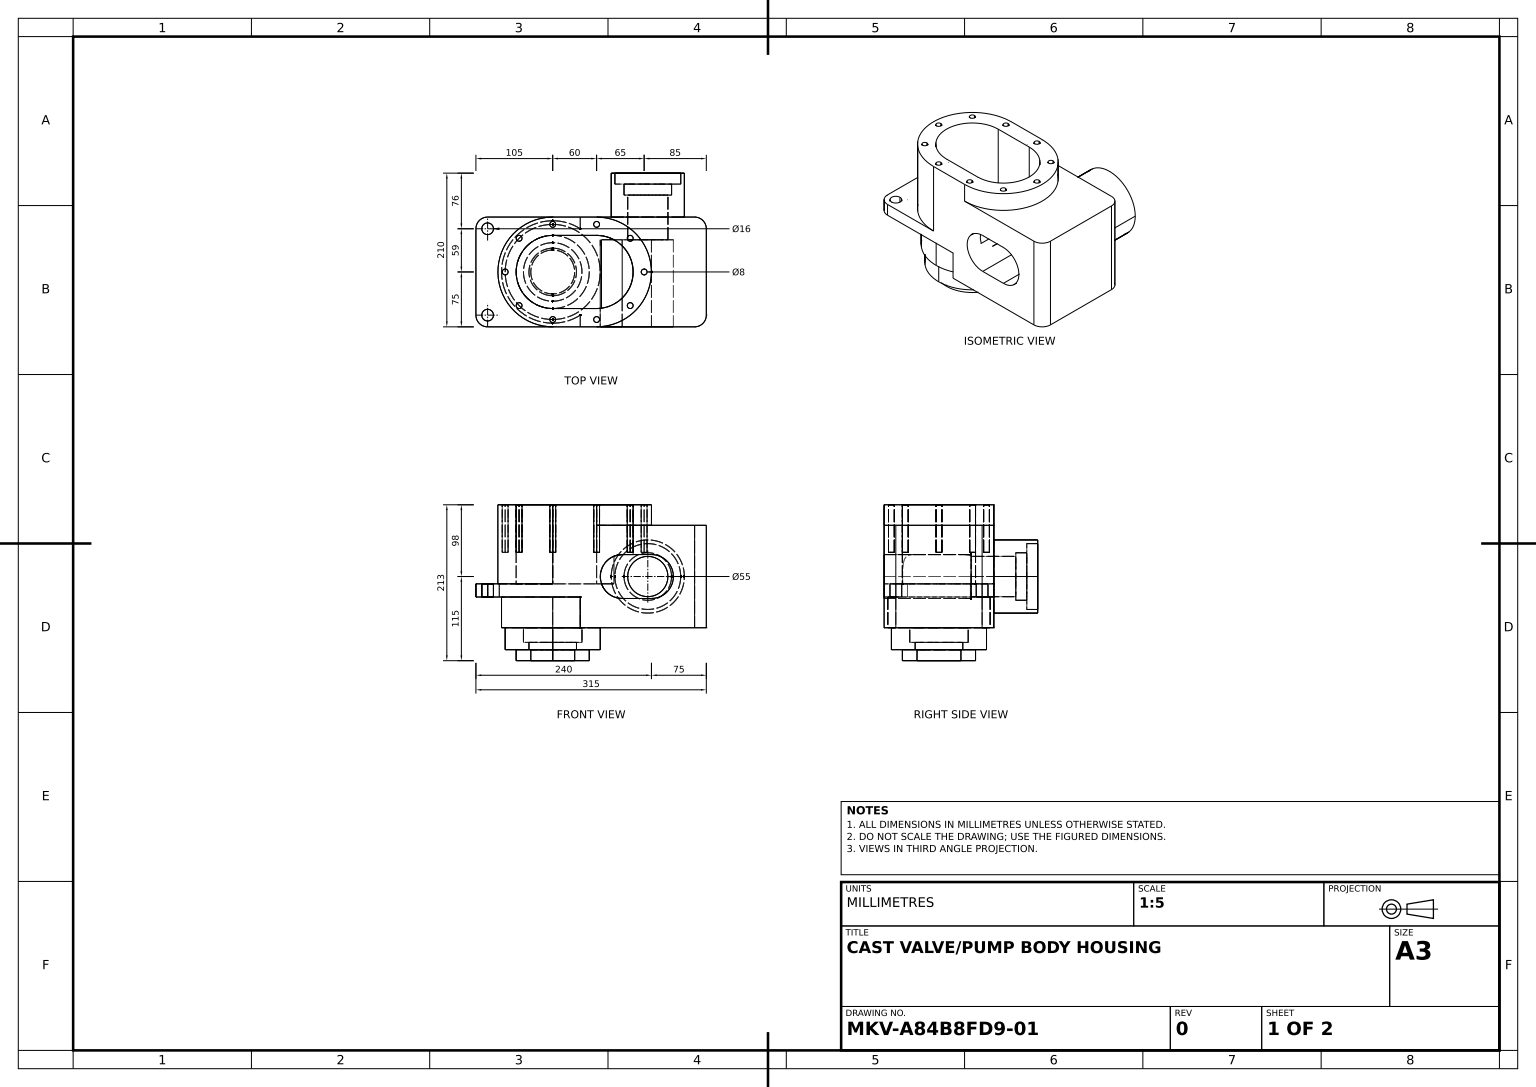
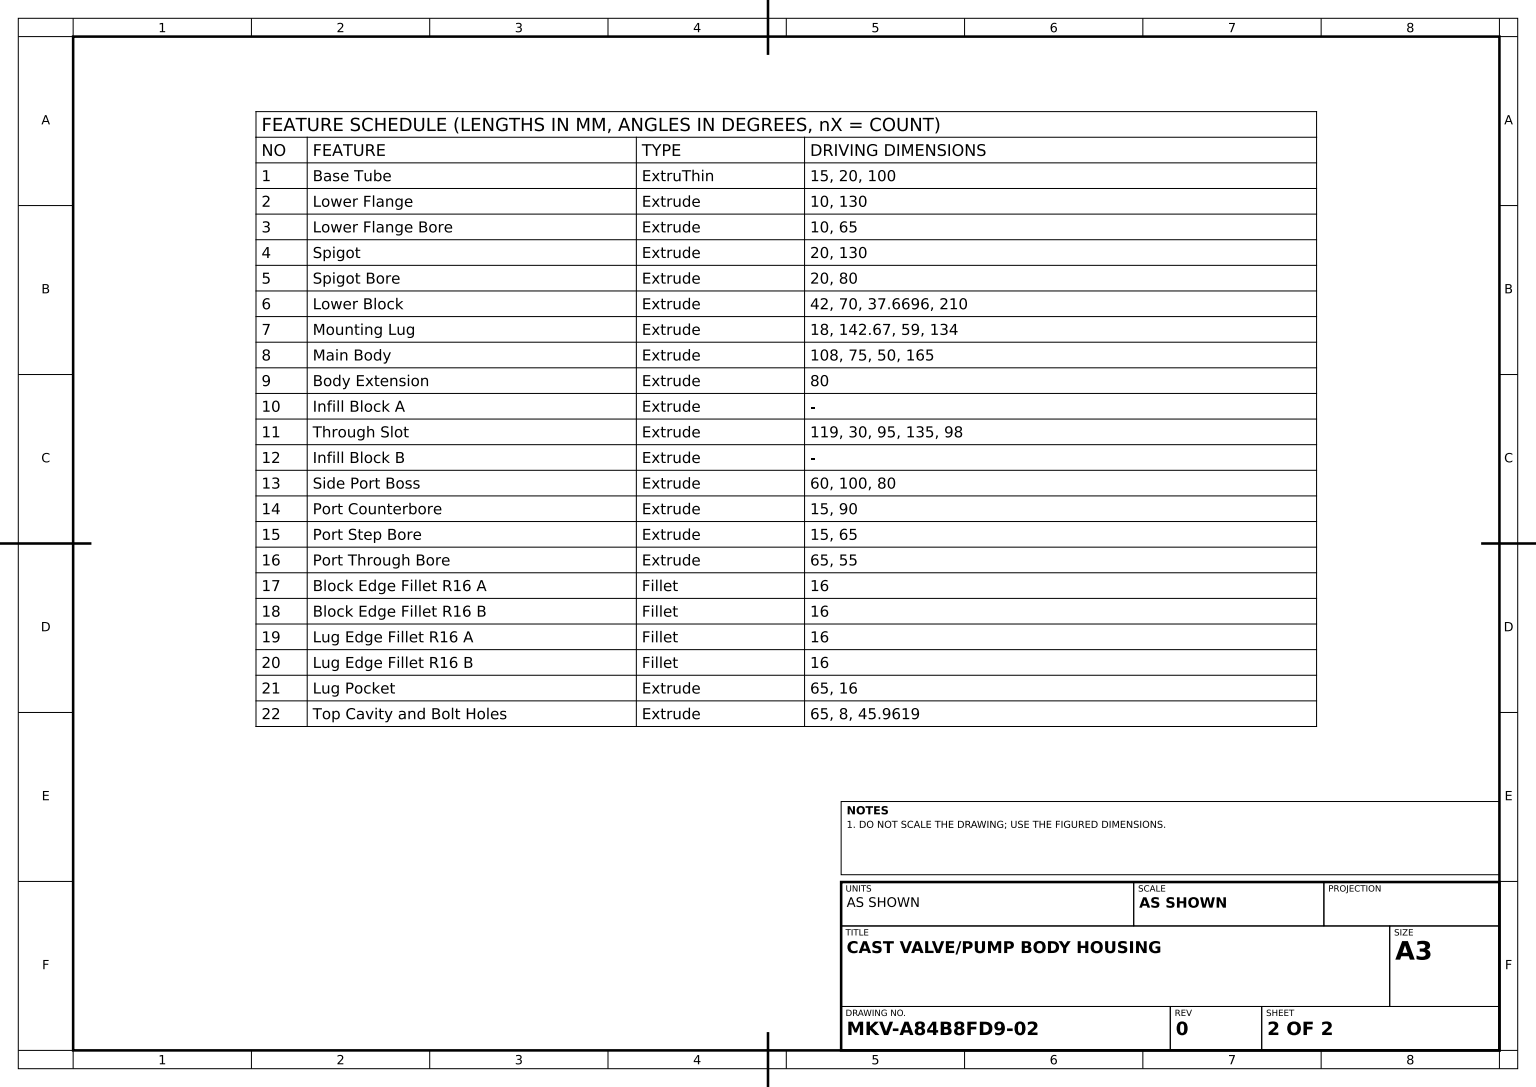
from build123d import *

# Parameters (mm, degrees)
BASE_TUBE_SKETCH_R                 = 50
BASE_TUBE_SKETCH_R_2               = 30
BASE_TUBE_DEPTH                    = 15
LOWER_FLANGE_SKETCH_R              = 65
LOWER_FLANGE_DEPTH                 = 10
LOWER_FLANGE_BORE_SKETCH_R         = 32.5
LOWER_FLANGE_BORE_DEPTH            = 10
SPIGOT_SKETCH_R                    = 65
SPIGOT_DEPTH                       = 20
SPIGOT_BORE_SKETCH_R               = 40
SPIGOT_BORE_DEPTH                  = 20
LOWER_BLOCK_DEPTH                  = 42
MOUNTING_LUG_DEPTH                 = 18
MAIN_BODY_DEPTH                    = 108
BODY_EXTENSION_DEPTH               = 80
INFILL_BLOCK_A_SKETCH_W            = 172.330383596
INFILL_BLOCK_A_SKETCH_H            = 42
INFILL_BLOCK_A_DEPTH               = 16
THROUGH_SLOT_DEPTH                 = 119
INFILL_BLOCK_B_SKETCH_W            = 172.330383596
INFILL_BLOCK_B_SKETCH_H            = 42
INFILL_BLOCK_B_DEPTH               = 16
SIDE_PORT_BOSS_SKETCH_R            = 50
SIDE_PORT_BOSS_DEPTH               = 60
PORT_COUNTERBORE_SKETCH_R          = 45
PORT_COUNTERBORE_DEPTH             = 15
PORT_STEP_BORE_SKETCH_R            = 32.5
PORT_STEP_BORE_DEPTH               = 15
PORT_THROUGH_BORE_SKETCH_R         = 27.5
PORT_THROUGH_BORE_DEPTH            = 65
BLOCK_EDGE_FILLET_R16_A_R          = 16
BLOCK_EDGE_FILLET_R16_B_R          = 16
LUG_EDGE_FILLET_R16_A_R            = 16
LUG_EDGE_FILLET_R16_B_R            = 16
LUG_POCKET_SKETCH_R                = 8
LUG_POCKET_DEPTH                   = 65
TOP_CAVITY_AND_BOLT_HOLES_SKETCH_R = 4
TOP_CAVITY_AND_BOLT_HOLES_DEPTH    = 65


with BuildPart() as part:
    # Base Tube Sketch → Base Tube (new body)
    with BuildSketch(Plane(origin=(0, 0, 0), x_dir=(1, 0, 0), z_dir=(0, 1, 0))):
        Circle(BASE_TUBE_SKETCH_R)
        Circle(BASE_TUBE_SKETCH_R_2, mode=Mode.SUBTRACT)
    extrude(amount=BASE_TUBE_DEPTH)

    # Lower Flange Sketch → Lower Flange (add)
    with BuildSketch(Plane(origin=(0, 15, 0), x_dir=(1, 0, 0), z_dir=(0, 1, 0))):
        with Locations(Location((0, 0, 0), (0, 0, 270))):
            Circle(LOWER_FLANGE_SKETCH_R)
    extrude(amount=LOWER_FLANGE_DEPTH)

    # Lower Flange Bore Sketch → Lower Flange Bore (cut)
    with BuildSketch(Plane(origin=(0, 25, 0), x_dir=(1, 0, 0), z_dir=(0, 1, 0))):
        with Locations(Location((0, 0, 0), (0, 0, 270))):
            Circle(LOWER_FLANGE_BORE_SKETCH_R)
    extrude(amount=-LOWER_FLANGE_BORE_DEPTH, mode=Mode.SUBTRACT)

    # Spigot Sketch → Spigot (add)
    with BuildSketch(Plane(origin=(0, 25, 0), x_dir=(1, 0, 0), z_dir=(0, 1, 0))):
        with Locations(Location((0, 0, 0), (0, 0, 270))):
            Circle(SPIGOT_SKETCH_R)
    extrude(amount=SPIGOT_DEPTH)

    # Spigot Bore Sketch → Spigot Bore (cut)
    with BuildSketch(Plane(origin=(0, 45, 0), x_dir=(1, 0, 0), z_dir=(0, 1, 0))):
        with Locations(Location((0, 0, 0), (0, 0, 270))):
            Circle(SPIGOT_BORE_SKETCH_R)
    extrude(amount=-SPIGOT_BORE_DEPTH, mode=Mode.SUBTRACT)

    # Lower Block Sketch → Lower Block (add)
    with BuildSketch(Plane(origin=(0, 45, 0), x_dir=(1, 0, 0), z_dir=(0, 1, 0))):
        with BuildLine():
            Line((37.669616404, 59), (210, 59))
            Line((210, 59), (210, -59))
            Line((210, -59), (37.669616404, -59))
            ThreePointArc((37.669616404, -59), (-70, 0), (37.669616404, 59))
        make_face()
    extrude(amount=LOWER_BLOCK_DEPTH)

    # Mounting Lug Sketch → Mounting Lug (add)
    with BuildSketch(Plane(origin=(0, 87, 0), x_dir=(1, 0, 0), z_dir=(0, 1, 0))):
        Polygon((-105, 0), (-105, 75), (210, 75), (210, -75), (-105, -75), align=None)
    extrude(amount=MOUNTING_LUG_DEPTH)

    # Main Body Sketch → Main Body (add)
    with BuildSketch(Plane(origin=(0, 105, 0), x_dir=(1, 0, 0), z_dir=(0, 1, 0))):
        with BuildLine():
            Line((0, 75), (60, 75))
            ThreePointArc((60, 75), (135, 0), (60, -75))
            Line((60, -75), (0, -75))
            ThreePointArc((0, -75), (-75, 0), (0, 75))
        make_face()
        with BuildLine():
            Line((0, 50), (60, 50))
            ThreePointArc((60, 50), (110, 0), (60, -50))
            Line((60, -50), (0, -50))
            ThreePointArc((0, -50), (-50, 0), (0, 50))
        make_face(mode=Mode.SUBTRACT)
    extrude(amount=MAIN_BODY_DEPTH)

    # Body Extension Sketch → Body Extension (add)
    with BuildSketch(Plane(origin=(0, 105, 0), x_dir=(1, 0, 0), z_dir=(0, 1, 0))):
        with BuildLine():
            Line((60, 75), (210, 75))
            Line((210, 75), (210, -75))
            Line((210, -75), (60, -75))
            ThreePointArc((60, -75), (135, 0), (60, 75))
        make_face()
    extrude(amount=BODY_EXTENSION_DEPTH)

    # Infill Block A Sketch → Infill Block A (add)
    with BuildSketch(Plane.XY.offset(59)):
        with Locations((123.834808202, 66)):
            Rectangle(INFILL_BLOCK_A_SKETCH_W, INFILL_BLOCK_A_SKETCH_H)
    extrude(amount=INFILL_BLOCK_A_DEPTH)

    # Through Slot Sketch → Through Slot (cut)
    with BuildSketch(Plane.XY.offset(75)):
        with BuildLine():
            Line((95, 145), (135, 145))
            ThreePointArc((135, 145), (165, 115), (135, 85))
            Line((135, 85), (95, 85))
            ThreePointArc((95, 85), (65, 115), (95, 145))
        make_face()
    extrude(amount=-THROUGH_SLOT_DEPTH, mode=Mode.SUBTRACT)

    # Infill Block B Sketch → Infill Block B (add)
    with BuildSketch(Plane(origin=(0, 0, -59), x_dir=(-1, 0, 0), z_dir=(0, 0, -1))):
        with Locations((-123.834808202, 66)):
            Rectangle(INFILL_BLOCK_B_SKETCH_W, INFILL_BLOCK_B_SKETCH_H)
    extrude(amount=INFILL_BLOCK_B_DEPTH)

    # Side Port Boss Sketch → Side Port Boss (add)
    with BuildSketch(Plane(origin=(0, 0, -75), x_dir=(-1, 0, 0), z_dir=(0, 0, -1))):
        with Locations(Location((-130, 115, 0), (0, 0, 180))):
            Circle(SIDE_PORT_BOSS_SKETCH_R)
    extrude(amount=SIDE_PORT_BOSS_DEPTH)

    # Port Counterbore Sketch → Port Counterbore (cut)
    with BuildSketch(Plane(origin=(0, 0, -135), x_dir=(-1, 0, 0), z_dir=(0, 0, -1))):
        with Locations((-130, 115)):
            Circle(PORT_COUNTERBORE_SKETCH_R)
    extrude(amount=-PORT_COUNTERBORE_DEPTH, mode=Mode.SUBTRACT)

    # Port Step Bore Sketch → Port Step Bore (cut)
    with BuildSketch(Plane(origin=(0, 0, -120), x_dir=(-1, 0, 0), z_dir=(0, 0, -1))):
        with Locations((-130, 115)):
            Circle(PORT_STEP_BORE_SKETCH_R)
    extrude(amount=-PORT_STEP_BORE_DEPTH, mode=Mode.SUBTRACT)

    # Port Through Bore Sketch → Port Through Bore (cut)
    with BuildSketch(Plane(origin=(0, 0, -105), x_dir=(-1, 0, 0), z_dir=(0, 0, -1))):
        with Locations((-130, 115)):
            Circle(PORT_THROUGH_BORE_SKETCH_R)
    extrude(amount=-PORT_THROUGH_BORE_DEPTH, mode=Mode.SUBTRACT)

    # Block Edge Fillet R16 A
    block_edge_fillet_r16_a_edges = [part.edges().sort_by_distance(p)[0] for p in [
        (210, 115, 75),
    ]]
    fillet(block_edge_fillet_r16_a_edges, radius=BLOCK_EDGE_FILLET_R16_A_R)

    # Block Edge Fillet R16 B
    block_edge_fillet_r16_b_edges = [part.edges().sort_by_distance(p)[0] for p in [
        (210, 115, -75),
    ]]
    fillet(block_edge_fillet_r16_b_edges, radius=BLOCK_EDGE_FILLET_R16_B_R)

    # Lug Edge Fillet R16 A
    lug_edge_fillet_r16_a_edges = [part.edges().sort_by_distance(p)[0] for p in [
        (-105, 96, 75),
    ]]
    fillet(lug_edge_fillet_r16_a_edges, radius=LUG_EDGE_FILLET_R16_A_R)

    # Lug Edge Fillet R16 B
    lug_edge_fillet_r16_b_edges = [part.edges().sort_by_distance(p)[0] for p in [
        (-105, 96, -75),
    ]]
    fillet(lug_edge_fillet_r16_b_edges, radius=LUG_EDGE_FILLET_R16_B_R)

    # Lug Pocket Sketch → Lug Pocket (cut)
    with BuildSketch(Plane(origin=(0, 105, 0), x_dir=(1, 0, 0), z_dir=(0, 1, 0))):
        with Locations(Location((-89, 59, 0), (0, 0, 270))):
            Circle(LUG_POCKET_SKETCH_R)
        with Locations(Location((-89, -59, 0), (0, 0, 270))):
            Circle(LUG_POCKET_SKETCH_R)
    extrude(amount=-LUG_POCKET_DEPTH, mode=Mode.SUBTRACT)

    # Top Cavity and Bolt Holes Sketch → Top Cavity and Bolt Holes (cut)
    with BuildSketch(Plane(origin=(0, 213, 0), x_dir=(1, 0, 0), z_dir=(0, 1, 0))):
        with Locations(Location((-65, 0, 0), (0, 0, 270))):
            Circle(TOP_CAVITY_AND_BOLT_HOLES_SKETCH_R)
        with Locations(Location((60, 65, 0), (0, 0, 270))):
            Circle(TOP_CAVITY_AND_BOLT_HOLES_SKETCH_R)
        with Locations(Location((105.961940777, 45.961940777, 0), (0, 0, 270))):
            Circle(TOP_CAVITY_AND_BOLT_HOLES_SKETCH_R)
        with Locations(Location((125, 0, 0), (0, 0, 270))):
            Circle(TOP_CAVITY_AND_BOLT_HOLES_SKETCH_R)
        with Locations(Location((105.961940777, -45.961940777, 0), (0, 0, 270))):
            Circle(TOP_CAVITY_AND_BOLT_HOLES_SKETCH_R)
        with Locations(Location((-45.961940777, -45.961940777, 0), (0, 0, 270))):
            Circle(TOP_CAVITY_AND_BOLT_HOLES_SKETCH_R)
        with Locations(Location((-45.961940777, 45.961940777, 0), (0, 0, 270))):
            Circle(TOP_CAVITY_AND_BOLT_HOLES_SKETCH_R)
        with Locations(Location((0, 65, 0), (0, 0, 270))):
            Circle(TOP_CAVITY_AND_BOLT_HOLES_SKETCH_R)
        with Locations(Location((60, -65, 0), (0, 0, 270))):
            Circle(TOP_CAVITY_AND_BOLT_HOLES_SKETCH_R)
        with Locations(Location((0, -65, 0), (0, 0, 270))):
            Circle(TOP_CAVITY_AND_BOLT_HOLES_SKETCH_R)
    extrude(amount=-TOP_CAVITY_AND_BOLT_HOLES_DEPTH, mode=Mode.SUBTRACT)


solid = part.part
